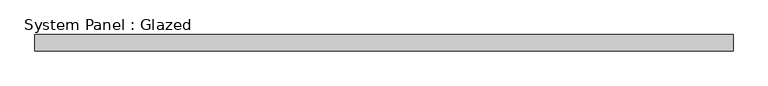
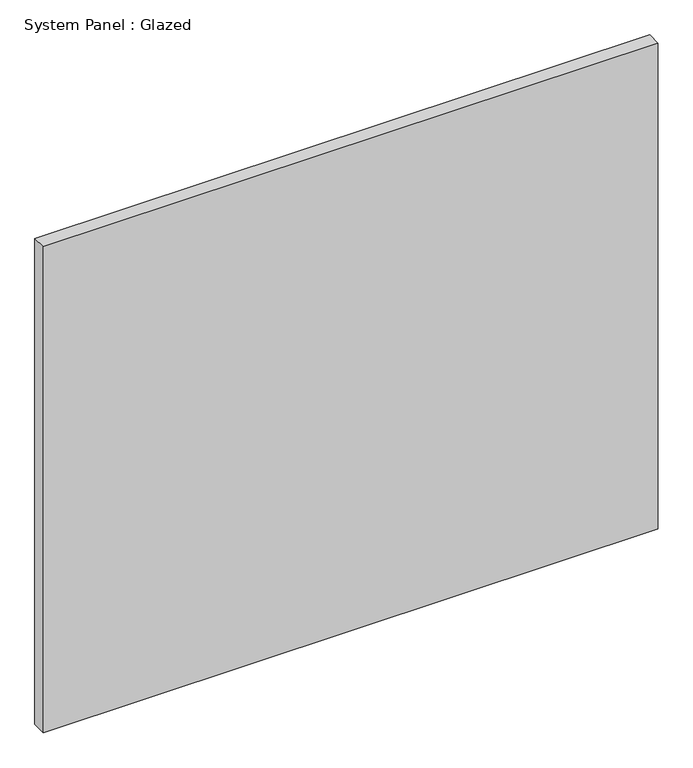
"""IFC4 building model written with IfcOpenShell, lengths in millimetres: plate geometry, System Panel : Glazed."""

from ifc_helpers import new_model, si_unit, origin, origin_with_axes, place, context, project, spatial, polyline, outline, extrude, source, transform, mapped, element, save


def system_panel_glazed_1bc24549(model_context):
    return source(origin(), model_context, "Body", "SweptSolid", [
        extrude(outline(polyline([(540.67075, 19.05), (-540.67075, 19.05), (-540.67075, 44.45), (540.67075, 44.45), (540.67075, 19.05)])), origin_with_axes(), (0.0, 0.0, 1.0), 903.5415),
    ])


if __name__ == "__main__":
    model = new_model("IFC4")
    model_context = context("Model", 3, world=origin())
    ifc_project = project(units=[si_unit("LENGTHUNIT", "METRE", prefix="MILLI")], contexts=[model_context])
    site = spatial("IfcSite", under=ifc_project)
    building = spatial("IfcBuilding", under=site)
    placement = place(None, origin())
    system_panel_glazed_shape = system_panel_glazed_1bc24549(model_context)
    element("IfcPlate", 1, ObjectType="System Panel : Glazed", at=placement, inside=building, context=model_context, shape_type="MappedRepresentation", body=[
        mapped(system_panel_glazed_shape, transform((0.0, 0.0, 0.0), x_axis=(1.0, 0.0, 0.0), y_axis=(0.0, 1.0, 0.0), z_axis=(0.0, 0.0, 1.0))),
    ])
    save(model, "model.ifc")

# Revit data of these elements
# Type "System Panel : Glazed"
#   Construction Type Id = "GSP4R"
#   Analytic Construction = "1/8 in Pilkington single glazing"
#   Visual Light Transmittance = 0.9
#   Solar Heat Gain Coefficient = 0.86
#   Heat Transfer Coefficient (U) = 1.18115 BTU/(h·ft²·°F)
#   Define Thermal Properties by = 1
# Element 1 (IfcPlate, "System Panel : Glazed")
#   Materials on its faces: "Glass"
# Materials
#   "Glass": class "Glass", colour RGB 0 128 192, transparency 0.75, Description = "Soda Lime Glass", Cost = 0
